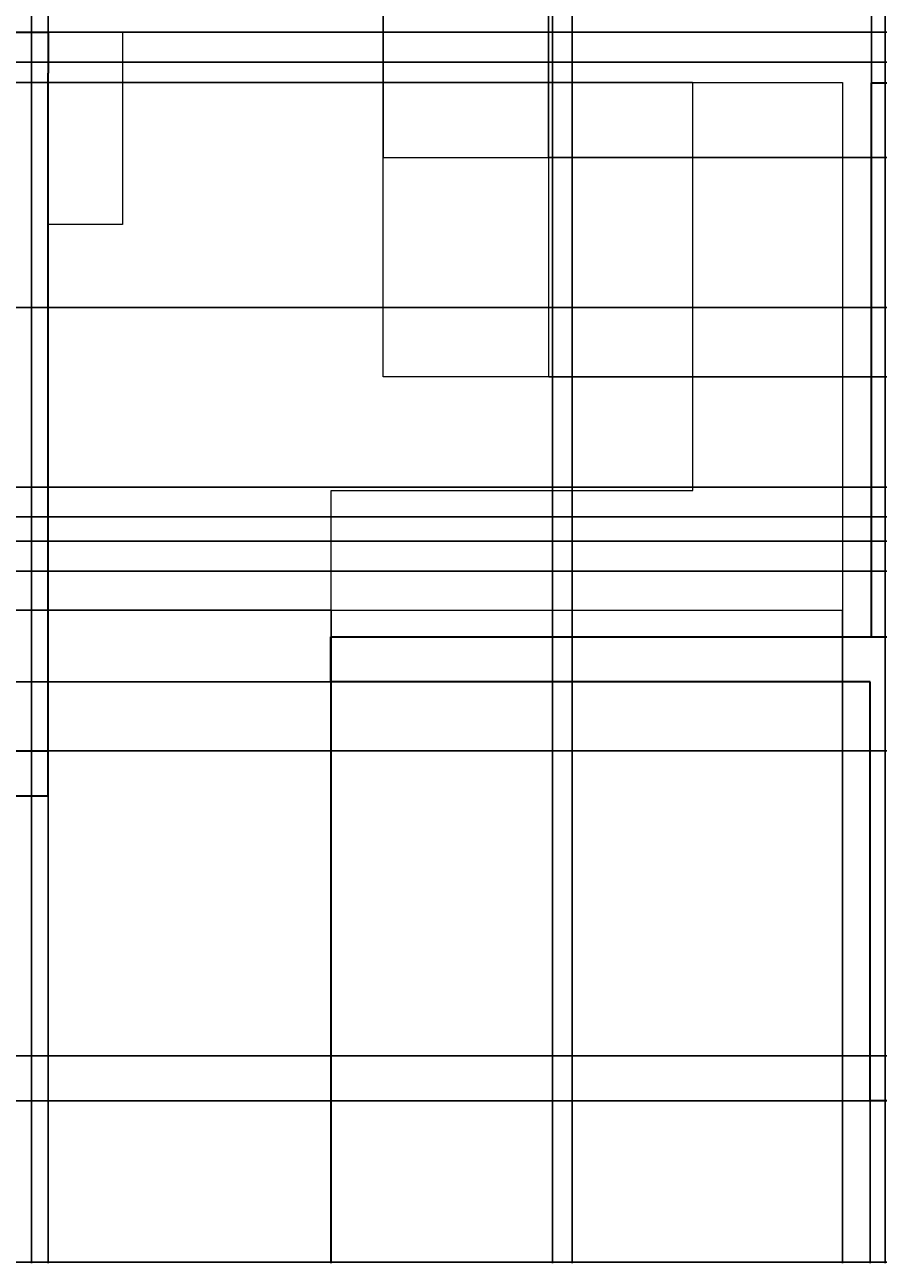
# Model space of a CAD drawing. Units: inches. Extents: x 1159 to 1869, y 2212 to 2738.
# Tile 3 of 5: x 1433 to 1604, y 2212 to 2460. Entities that reach past the tile are written whole.
import ezdxf

# ---------------------------------------------------------------- set-up
doc = ezdxf.new("R2010")
doc.units = ezdxf.units.IN
for name, color, linetype, lineweight in [('A-ANNO-DIMS', 2, 'Continuous', 18), ('A-FLOR-CASE', 30, 'Continuous', 18), ('A-FURN', 8, 'Continuous', 18), ('A-WALL', 7, 'Continuous', 35)]:
    doc.layers.add(name, color=color, linetype=linetype, lineweight=lineweight)
doc.styles.get("Standard").update_dxf_attribs({"font": 'arial.ttf'})
doc.dimstyles.get("Standard").update_dxf_attribs({"dimtxt": 0.18, "dimasz": 0.18, "dimexe": 0.18, "dimexo": 0.0625, "dimgap": 0.09, "dimtad": 0, "dimtih": 1, "dimtoh": 1, "dimdec": 4, "dimzin": 0, "dimdsep": 46, "dimtxsty": 'Standard', "dimcen": 0.09, "dimadec": 0, "dimazin": 0, "dimtfac": 1, "dimtdec": 4, "dimtofl": 0, "dimtmove": 0, "dimatfit": 3, "dimfxl": 1, "dimtolj": 1, "dimtzin": 0, "dimarcsym": 0})

# ---------------------------------------------------------------- blocks, each defined once
blk = doc.blocks.new('*D26')
at = {"layer": 'A-ANNO-DIMS', "color": 0, "lineweight": -2, "transparency": 16777216}
for p, q in [((1191.4, 2305.14), (1191.4, 2211.56)), ((1437.74, 2305.14), (1437.74, 2211.56)), ((1191.58, 2211.74), (1314.11, 2211.74)), ((1437.56, 2211.74), (1315.04, 2211.74))]:
    blk.add_line(p, q, dxfattribs=at)
at = {"layer": 'A-ANNO-DIMS', "color": 0, "transparency": 16777216}
for points in [[(1191.58, 2211.77), (1191.58, 2211.71), (1191.4, 2211.74)], [(1437.56, 2211.77), (1437.56, 2211.71), (1437.74, 2211.74)]]:
    blk.add_solid(points, dxfattribs=at)
at = {"layer": 'Defpoints', "color": 0, "transparency": 16777216}
for p in [(1191.4, 2305.21), (1437.74, 2305.21), (1437.74, 2211.74)]:
    blk.add_point(p, dxfattribs=at)
at = {"layer": 'A-ANNO-DIMS', "color": 0, "transparency": 16777216, "insert": (1314.57, 2211.74), "char_height": 0.18, "attachment_point": 5}
blk.add_mtext('\\A1;246.34', dxfattribs=at)
blk = doc.blocks.new('*D27')
at = {"layer": 'A-ANNO-DIMS', "color": 0, "lineweight": -2, "transparency": 16777216}
for p, q in [((1437.74, 2305.14), (1437.74, 2211.56)), ((1602.4, 2244.01), (1602.4, 2211.56)), ((1437.92, 2211.74), (1519.62, 2211.74)), ((1602.22, 2211.74), (1520.53, 2211.74))]:
    blk.add_line(p, q, dxfattribs=at)
at = {"layer": 'A-ANNO-DIMS', "color": 0, "transparency": 16777216}
for points in [[(1437.92, 2211.77), (1437.92, 2211.71), (1437.74, 2211.74)], [(1602.22, 2211.77), (1602.22, 2211.71), (1602.4, 2211.74)]]:
    blk.add_solid(points, dxfattribs=at)
at = {"layer": 'Defpoints', "color": 0, "transparency": 16777216}
for p in [(1437.74, 2305.21), (1602.4, 2244.08), (1602.4, 2211.74)]:
    blk.add_point(p, dxfattribs=at)
at = {"layer": 'A-ANNO-DIMS', "color": 0, "transparency": 16777216, "insert": (1520.07, 2211.74), "char_height": 0.18, "attachment_point": 5}
blk.add_mtext('\\A1;164.66', dxfattribs=at)
blk = doc.blocks.new('*D28')
at = {"layer": 'A-ANNO-DIMS', "color": 0, "lineweight": -2, "transparency": 16777216}
for p, q in [((1602.4, 2244.01), (1602.4, 2211.56)), ((1752.4, 2244.01), (1752.4, 2211.56)), ((1602.58, 2211.74), (1677.12, 2211.74)), ((1752.22, 2211.74), (1677.68, 2211.74))]:
    blk.add_line(p, q, dxfattribs=at)
at = {"layer": 'A-ANNO-DIMS', "color": 0, "transparency": 16777216}
for points in [[(1602.58, 2211.77), (1602.58, 2211.71), (1602.4, 2211.74)], [(1752.22, 2211.77), (1752.22, 2211.71), (1752.4, 2211.74)]]:
    blk.add_solid(points, dxfattribs=at)
at = {"layer": 'Defpoints', "color": 0, "transparency": 16777216}
for p in [(1602.4, 2244.08), (1752.4, 2244.08), (1752.4, 2211.74)]:
    blk.add_point(p, dxfattribs=at)
at = {"layer": 'A-ANNO-DIMS', "color": 0, "transparency": 16777216, "insert": (1677.4, 2211.74), "char_height": 0.18, "attachment_point": 5}
blk.add_mtext('\\A1;150', dxfattribs=at)
blk = doc.blocks.new('*D42')
at = {"layer": 'A-ANNO-DIMS', "color": 0, "lineweight": -2, "transparency": 16777216}
for p, q in [((1200.46, 2452.21), (1868.92, 2452.21)), ((1868.74, 2452.03), (1868.74, 2404.39)), ((1868.74, 2356.39), (1868.74, 2404.02)), ((1200.46, 2356.21), (1868.92, 2356.21))]:
    blk.add_line(p, q, dxfattribs=at)
at = {"layer": 'A-ANNO-DIMS', "color": 0, "transparency": 16777216}
for points in [[(1868.71, 2452.03), (1868.77, 2452.03), (1868.74, 2452.21)], [(1868.71, 2356.39), (1868.77, 2356.39), (1868.74, 2356.21)]]:
    blk.add_solid(points, dxfattribs=at)
at = {"layer": 'Defpoints', "color": 0, "transparency": 16777216}
for p in [(1200.4, 2452.21), (1868.74, 2452.21), (1200.4, 2356.21)]:
    blk.add_point(p, dxfattribs=at)
at = {"layer": 'A-ANNO-DIMS', "color": 0, "transparency": 16777216, "insert": (1868.74, 2404.21), "char_height": 0.18, "attachment_point": 5}
blk.add_mtext('\\A1;96', dxfattribs=at)
blk = doc.blocks.new('*D45')
at = {"layer": 'A-ANNO-DIMS', "color": 0, "lineweight": -2, "transparency": 16777216}
for p, q in [((1494.4, 2328.01), (1494.4, 2211.56)), ((1602.4, 2328.01), (1602.4, 2211.56)), ((1494.58, 2211.74), (1548.12, 2211.74)), ((1602.22, 2211.74), (1548.68, 2211.74))]:
    blk.add_line(p, q, dxfattribs=at)
at = {"layer": 'A-ANNO-DIMS', "color": 0, "transparency": 16777216}
for points in [[(1494.58, 2211.77), (1494.58, 2211.71), (1494.4, 2211.74)], [(1602.22, 2211.77), (1602.22, 2211.71), (1602.4, 2211.74)]]:
    blk.add_solid(points, dxfattribs=at)
at = {"layer": 'Defpoints', "color": 0, "transparency": 16777216}
for p in [(1494.4, 2328.08), (1602.4, 2328.08), (1602.4, 2211.74)]:
    blk.add_point(p, dxfattribs=at)
at = {"layer": 'A-ANNO-DIMS', "color": 0, "transparency": 16777216, "insert": (1548.4, 2211.74), "char_height": 0.18, "attachment_point": 5}
blk.add_mtext('\\A1;108', dxfattribs=at)
blk = doc.blocks.new('*D46')
at = {"layer": 'A-ANNO-DIMS', "color": 0, "lineweight": -2, "transparency": 16777216}
for p, q in [((1602.34, 2328.08), (1158.88, 2328.08)), ((1159.06, 2327.9), (1159.06, 2286.26)), ((1159.06, 2244.26), (1159.06, 2285.89)), ((1602.34, 2244.08), (1158.88, 2244.08))]:
    blk.add_line(p, q, dxfattribs=at)
at = {"layer": 'A-ANNO-DIMS', "color": 0, "transparency": 16777216}
for points in [[(1159.03, 2327.9), (1159.09, 2327.9), (1159.06, 2328.08)], [(1159.03, 2244.26), (1159.09, 2244.26), (1159.06, 2244.08)]]:
    blk.add_solid(points, dxfattribs=at)
at = {"layer": 'Defpoints', "color": 0, "transparency": 16777216}
for p in [(1159.06, 2328.08), (1602.4, 2328.08), (1602.4, 2244.08)]:
    blk.add_point(p, dxfattribs=at)
at = {"layer": 'A-ANNO-DIMS', "color": 0, "transparency": 16777216, "insert": (1159.06, 2286.08), "char_height": 0.18, "attachment_point": 5}
blk.add_mtext('\\A1;84', dxfattribs=at)
blk = doc.blocks.new('*D48')
at = {"layer": 'A-ANNO-DIMS', "color": 0, "lineweight": -2, "transparency": 16777216}
for p, q in [((1437.74, 2458.27), (1437.74, 2738.15)), ((1437.92, 2737.97), (1519.76, 2737.97)), ((1602.5, 2737.97), (1520.67, 2737.97)), ((1602.68, 2448.14), (1602.68, 2738.15))]:
    blk.add_line(p, q, dxfattribs=at)
at = {"layer": 'A-ANNO-DIMS', "color": 0, "transparency": 16777216}
for points in [[(1437.92, 2738), (1437.92, 2737.94), (1437.74, 2737.97)], [(1602.5, 2738), (1602.5, 2737.94), (1602.68, 2737.97)]]:
    blk.add_solid(points, dxfattribs=at)
at = {"layer": 'Defpoints', "color": 0, "transparency": 16777216}
for p in [(1602.68, 2737.97), (1437.74, 2458.21), (1602.68, 2448.08)]:
    blk.add_point(p, dxfattribs=at)
at = {"layer": 'A-ANNO-DIMS', "color": 0, "transparency": 16777216, "insert": (1520.21, 2737.97), "char_height": 0.18, "attachment_point": 5}
blk.add_mtext('\\A1;164.94', dxfattribs=at)
blk = doc.blocks.new('*D53')
at = {"layer": 'A-ANNO-DIMS', "color": 0, "lineweight": -2, "transparency": 16777216}
for p, q in [((1425.46, 2504.63), (1868.92, 2504.63)), ((1868.74, 2504.45), (1868.74, 2481.6)), ((1868.74, 2458.39), (1868.74, 2481.24)), ((1428.81, 2458.21), (1868.92, 2458.21))]:
    blk.add_line(p, q, dxfattribs=at)
at = {"layer": 'A-ANNO-DIMS', "color": 0, "transparency": 16777216}
for points in [[(1868.71, 2504.45), (1868.77, 2504.45), (1868.74, 2504.63)], [(1868.71, 2458.39), (1868.77, 2458.39), (1868.74, 2458.21)]]:
    blk.add_solid(points, dxfattribs=at)
at = {"layer": 'Defpoints', "color": 0, "transparency": 16777216}
for p in [(1425.4, 2504.63), (1868.74, 2504.63), (1428.74, 2458.21)]:
    blk.add_point(p, dxfattribs=at)
at = {"layer": 'A-ANNO-DIMS', "color": 0, "transparency": 16777216, "insert": (1868.74, 2481.42), "char_height": 0.18, "attachment_point": 5}
blk.add_mtext('\\A1;46.42', dxfattribs=at)
blk = doc.blocks.new('*D54')
at = {"layer": 'A-ANNO-DIMS', "color": 0, "lineweight": -2, "transparency": 16777216}
for p, q in [((1437.68, 2305.21), (1158.88, 2305.21)), ((1159.06, 2305.03), (1159.06, 2274.82)), ((1159.06, 2244.26), (1159.06, 2274.46)), ((1602.34, 2244.08), (1158.88, 2244.08))]:
    blk.add_line(p, q, dxfattribs=at)
at = {"layer": 'A-ANNO-DIMS', "color": 0, "transparency": 16777216}
for points in [[(1159.03, 2305.03), (1159.09, 2305.03), (1159.06, 2305.21)], [(1159.03, 2244.26), (1159.09, 2244.26), (1159.06, 2244.08)]]:
    blk.add_solid(points, dxfattribs=at)
at = {"layer": 'Defpoints', "color": 0, "transparency": 16777216}
for p in [(1437.74, 2305.21), (1159.06, 2244.08), (1602.4, 2244.08)]:
    blk.add_point(p, dxfattribs=at)
at = {"layer": 'A-ANNO-DIMS', "color": 0, "transparency": 16777216, "insert": (1159.06, 2274.64), "char_height": 0.18, "attachment_point": 5}
blk.add_mtext('\\A1;61.13', dxfattribs=at)
blk = doc.blocks.new('*D55')
at = {"layer": 'A-ANNO-DIMS', "color": 0, "lineweight": -2, "transparency": 16777216}
for p, q in [((1494.46, 2342.31), (1494.46, 2211.56)), ((1596.87, 2342.31), (1596.87, 2211.56)), ((1494.64, 2211.74), (1545.28, 2211.74)), ((1596.69, 2211.74), (1546.05, 2211.74))]:
    blk.add_line(p, q, dxfattribs=at)
at = {"layer": 'A-ANNO-DIMS', "color": 0, "transparency": 16777216}
for points in [[(1494.64, 2211.77), (1494.64, 2211.71), (1494.46, 2211.74)], [(1596.69, 2211.77), (1596.69, 2211.71), (1596.87, 2211.74)]]:
    blk.add_solid(points, dxfattribs=at)
at = {"layer": 'Defpoints', "color": 0, "transparency": 16777216}
for p in [(1494.46, 2342.38), (1596.87, 2342.38), (1596.87, 2211.74)]:
    blk.add_point(p, dxfattribs=at)
at = {"layer": 'A-ANNO-DIMS', "color": 0, "transparency": 16777216, "insert": (1545.66, 2211.74), "char_height": 0.18, "attachment_point": 5}
blk.add_mtext('\\A1;102.4', dxfattribs=at)
blk = doc.blocks.new('*D56')
at = {"layer": 'A-ANNO-DIMS', "color": 0, "lineweight": -2, "transparency": 16777216}
for p, q in [((1566.83, 2448.11), (1158.88, 2448.11)), ((1159.06, 2447.93), (1159.06, 2395.42)), ((1159.06, 2342.56), (1159.06, 2395.06)), ((1494.4, 2342.38), (1158.88, 2342.38))]:
    blk.add_line(p, q, dxfattribs=at)
at = {"layer": 'A-ANNO-DIMS', "color": 0, "transparency": 16777216}
for points in [[(1159.03, 2447.93), (1159.09, 2447.93), (1159.06, 2448.11)], [(1159.03, 2342.56), (1159.09, 2342.56), (1159.06, 2342.38)]]:
    blk.add_solid(points, dxfattribs=at)
at = {"layer": 'Defpoints', "color": 0, "transparency": 16777216}
for p in [(1566.9, 2448.11), (1159.06, 2342.38), (1494.46, 2342.38)]:
    blk.add_point(p, dxfattribs=at)
at = {"layer": 'A-ANNO-DIMS', "color": 0, "transparency": 16777216, "insert": (1159.06, 2395.24), "char_height": 0.18, "attachment_point": 5}
blk.add_mtext('\\A1;105.73', dxfattribs=at)
blk = doc.blocks.new('*D57')
at = {"layer": 'A-ANNO-DIMS', "color": 0, "lineweight": -2, "transparency": 16777216}
for p, q in [((1504.87, 2433.16), (1504.87, 2738.15)), ((1505.05, 2737.97), (1521.04, 2737.97)), ((1537.79, 2737.97), (1521.8, 2737.97)), ((1537.97, 2433.16), (1537.97, 2738.15))]:
    blk.add_line(p, q, dxfattribs=at)
at = {"layer": 'A-ANNO-DIMS', "color": 0, "transparency": 16777216}
for points in [[(1505.05, 2738), (1505.05, 2737.94), (1504.87, 2737.97)], [(1537.79, 2738), (1537.79, 2737.94), (1537.97, 2737.97)]]:
    blk.add_solid(points, dxfattribs=at)
at = {"layer": 'Defpoints', "color": 0, "transparency": 16777216}
for p in [(1537.97, 2737.97), (1504.87, 2433.09), (1537.97, 2433.09)]:
    blk.add_point(p, dxfattribs=at)
at = {"layer": 'A-ANNO-DIMS', "color": 0, "transparency": 16777216, "insert": (1521.42, 2737.97), "char_height": 0.18, "attachment_point": 5}
blk.add_mtext('\\A1;33.11', dxfattribs=at)
blk = doc.blocks.new('*D58')
at = {"layer": 'A-ANNO-DIMS', "color": 0, "lineweight": -2, "transparency": 16777216}
for p, q in [((1538.03, 2433.09), (1868.92, 2433.09)), ((1868.74, 2432.91), (1868.74, 2411.32)), ((1868.74, 2389.36), (1868.74, 2410.95)), ((1538.03, 2389.18), (1868.92, 2389.18))]:
    blk.add_line(p, q, dxfattribs=at)
at = {"layer": 'A-ANNO-DIMS', "color": 0, "transparency": 16777216}
for points in [[(1868.71, 2432.91), (1868.77, 2432.91), (1868.74, 2433.09)], [(1868.71, 2389.36), (1868.77, 2389.36), (1868.74, 2389.18)]]:
    blk.add_solid(points, dxfattribs=at)
at = {"layer": 'Defpoints', "color": 0, "transparency": 16777216}
for p in [(1537.97, 2433.09), (1868.74, 2433.09), (1537.97, 2389.18)]:
    blk.add_point(p, dxfattribs=at)
at = {"layer": 'A-ANNO-DIMS', "color": 0, "transparency": 16777216, "insert": (1868.74, 2411.14), "char_height": 0.18, "attachment_point": 5}
blk.add_mtext('\\A1;43.92', dxfattribs=at)
blk = doc.blocks.new('*D64')
at = {"layer": 'A-ANNO-DIMS', "color": 0, "lineweight": -2, "transparency": 16777216}
for p, q in [((1434.4, 2660.2), (1434.4, 2211.56)), ((1538.82, 2660.2), (1538.82, 2211.56)), ((1434.58, 2211.74), (1486.15, 2211.74)), ((1538.64, 2211.74), (1487.06, 2211.74))]:
    blk.add_line(p, q, dxfattribs=at)
at = {"layer": 'A-ANNO-DIMS', "color": 0, "transparency": 16777216}
for points in [[(1434.58, 2211.77), (1434.58, 2211.71), (1434.4, 2211.74)], [(1538.64, 2211.77), (1538.64, 2211.71), (1538.82, 2211.74)]]:
    blk.add_solid(points, dxfattribs=at)
at = {"layer": 'Defpoints', "color": 0, "transparency": 16777216}
for p in [(1434.4, 2660.26), (1538.82, 2660.26), (1434.4, 2211.74)]:
    blk.add_point(p, dxfattribs=at)
at = {"layer": 'A-ANNO-DIMS', "color": 0, "transparency": 16777216, "insert": (1486.61, 2211.74), "char_height": 0.18, "attachment_point": 5}
blk.add_mtext('\\A1;104.42', dxfattribs=at)
blk = doc.blocks.new('*D65')
at = {"layer": 'A-ANNO-DIMS', "color": 0, "lineweight": -2, "transparency": 16777216}
for p, q in [((1542.76, 2504.57), (1542.76, 2211.56)), ((1605.4, 2504.57), (1605.4, 2211.56)), ((1542.94, 2211.74), (1573.69, 2211.74)), ((1605.22, 2211.74), (1574.48, 2211.74))]:
    blk.add_line(p, q, dxfattribs=at)
at = {"layer": 'A-ANNO-DIMS', "color": 0, "transparency": 16777216}
for points in [[(1542.94, 2211.77), (1542.94, 2211.71), (1542.76, 2211.74)], [(1605.22, 2211.77), (1605.22, 2211.71), (1605.4, 2211.74)]]:
    blk.add_solid(points, dxfattribs=at)
at = {"layer": 'Defpoints', "color": 0, "transparency": 16777216}
for p in [(1542.76, 2504.63), (1605.4, 2504.63), (1605.4, 2211.74)]:
    blk.add_point(p, dxfattribs=at)
at = {"layer": 'A-ANNO-DIMS', "color": 0, "transparency": 16777216, "insert": (1574.08, 2211.74), "char_height": 0.18, "attachment_point": 5}
blk.add_mtext('\\A1;62.64', dxfattribs=at)
blk = doc.blocks.new('*D67')
at = {"layer": 'A-ANNO-DIMS', "color": 0, "lineweight": -2, "transparency": 16777216}
for p, q in [((1665.34, 2403.08), (1158.88, 2403.08)), ((1159.06, 2402.9), (1159.06, 2385.26)), ((1159.06, 2367.26), (1159.06, 2384.89)), ((1665.34, 2367.08), (1158.88, 2367.08))]:
    blk.add_line(p, q, dxfattribs=at)
at = {"layer": 'A-ANNO-DIMS', "color": 0, "transparency": 16777216}
for points in [[(1159.03, 2402.9), (1159.09, 2402.9), (1159.06, 2403.08)], [(1159.03, 2367.26), (1159.09, 2367.26), (1159.06, 2367.08)]]:
    blk.add_solid(points, dxfattribs=at)
at = {"layer": 'Defpoints', "color": 0, "transparency": 16777216}
for p in [(1159.06, 2403.08), (1665.4, 2403.08), (1665.4, 2367.08)]:
    blk.add_point(p, dxfattribs=at)
at = {"layer": 'A-ANNO-DIMS', "color": 0, "transparency": 16777216, "insert": (1159.06, 2385.08), "char_height": 0.18, "attachment_point": 5}
blk.add_mtext('\\A1;36', dxfattribs=at)
blk = doc.blocks.new('*D74')
at = {"layer": 'A-ANNO-DIMS', "color": 0, "lineweight": -2, "transparency": 16777216}
for p, q in [((1743.34, 2361.08), (1158.88, 2361.08)), ((1159.06, 2360.9), (1159.06, 2307.26)), ((1159.06, 2253.26), (1159.06, 2306.89)), ((1743.34, 2253.08), (1158.88, 2253.08))]:
    blk.add_line(p, q, dxfattribs=at)
at = {"layer": 'A-ANNO-DIMS', "color": 0, "transparency": 16777216}
for points in [[(1159.03, 2360.9), (1159.09, 2360.9), (1159.06, 2361.08)], [(1159.03, 2253.26), (1159.09, 2253.26), (1159.06, 2253.08)]]:
    blk.add_solid(points, dxfattribs=at)
at = {"layer": 'Defpoints', "color": 0, "transparency": 16777216}
for p in [(1159.06, 2361.08), (1743.4, 2361.08), (1743.4, 2253.08)]:
    blk.add_point(p, dxfattribs=at)
at = {"layer": 'A-ANNO-DIMS', "color": 0, "transparency": 16777216, "insert": (1159.06, 2307.08), "char_height": 0.18, "attachment_point": 5}
blk.add_mtext('\\A1;108', dxfattribs=at)
blk = doc.blocks.new('*D75')
at = {"layer": 'A-ANNO-DIMS', "color": 0, "lineweight": -2, "transparency": 16777216}
for p, q in [((1227.43, 2350.21), (1868.92, 2350.21)), ((1868.74, 2350.03), (1868.74, 2332.39)), ((1868.74, 2314.39), (1868.74, 2332.02)), ((1227.43, 2314.21), (1868.92, 2314.21))]:
    blk.add_line(p, q, dxfattribs=at)
at = {"layer": 'A-ANNO-DIMS', "color": 0, "transparency": 16777216}
for points in [[(1868.71, 2350.03), (1868.77, 2350.03), (1868.74, 2350.21)], [(1868.71, 2314.39), (1868.77, 2314.39), (1868.74, 2314.21)]]:
    blk.add_solid(points, dxfattribs=at)
at = {"layer": 'Defpoints', "color": 0, "transparency": 16777216}
for p in [(1227.37, 2350.21), (1868.74, 2350.21), (1227.37, 2314.21)]:
    blk.add_point(p, dxfattribs=at)
at = {"layer": 'A-ANNO-DIMS', "color": 0, "transparency": 16777216, "insert": (1868.74, 2332.21), "char_height": 0.18, "attachment_point": 5}
blk.add_mtext('\\A1;36', dxfattribs=at)

msp = doc.modelspace()

# ---------------------------------------------------------------- linework, layer by layer
at = {"layer": 'A-FLOR-CASE'}
for p, q in [((1437.7443, 2458.2064), (1452.6751, 2458.2064)), ((1452.6751, 2458.2064), (1452.6751, 2419.6842)), ((1452.6751, 2419.6842), (1437.7443, 2419.6842))]:
    msp.add_line(p, q, dxfattribs=at)
at = {"layer": 'A-FURN'}
for p, q in [((1566.895, 2366.3753), (1566.895, 2448.1096)), ((1566.895, 2448.1096), (1596.8651, 2448.1096)), ((1596.8651, 2448.1096), (1596.8651, 2342.3753)), ((1494.4613, 2342.3753), (1494.4613, 2366.3753)), ((1494.4613, 2366.3753), (1566.895, 2366.3753)), ((1596.8651, 2342.3753), (1494.4613, 2342.3753))]:
    msp.add_line(p, q, dxfattribs=at)
msp.add_lwpolyline([(1504.8654, 2433.0936), (1537.9722, 2433.0936), (1537.9722, 2389.1774), (1504.8654, 2389.1774)], close=True, dxfattribs=at)
at = {"layer": 'A-WALL'}
for p, q in [((1428.7443, 2458.2064), (1437.7443, 2458.2064)), ((1437.7443, 2458.2064), (1437.7443, 2449.977)), ((1437.7443, 2314.2064), (1437.7443, 2449.977)), ((1602.6806, 2337.0757), (1602.6806, 2448.0757)), ((1602.6806, 2448.0757), (1632.6806, 2448.0757)), ((1494.4011, 2328.0757), (1494.4011, 2337.0757)), ((1494.4011, 2337.0757), (1611.4011, 2337.0757)), ((1602.4011, 2328.0757), (1494.4011, 2328.0757)), ((1602.4011, 2244.0757), (1602.4011, 2328.0757)), ((1200.4011, 2314.2064), (1437.7443, 2314.2064)), ((1437.7443, 2305.2064), (1437.7443, 2314.2064)), ((1191.4011, 2305.2064), (1437.7443, 2305.2064)), ((1614.4011, 2244.0757), (1602.4011, 2244.0757))]:
    msp.add_line(p, q, dxfattribs=at)

# ---------------------------------------------------------------- dimensions: what is measured, and where the dimension line sits
at = {"layer": 'A-ANNO-DIMS'}
for base, p1, p2, override, picture, middle in [((1602.6806, 2737.9679), (1437.7443, 2458.2064), (1602.6806, 2448.0757), {"dimdec": 2, "dimlfac": 1, "dimrnd": 0, "dimzin": 0, "dimdsep": 46, "dimlunit": 2}, '*D48', (1520.2124, 2737.9679)), ((1537.9722, 2737.9679), (1504.8654, 2433.0936), (1537.9722, 2433.0936), {"dimdec": 2, "dimlfac": 1, "dimrnd": 0, "dimzin": 0, "dimdsep": 46, "dimlunit": 2}, '*D57', (1521.4188, 2737.9679)), ((1434.4011, 2211.7357), (1538.817, 2660.2597), (1434.4011, 2660.2597), {"dimdec": 2, "dimlfac": 1, "dimrnd": 0, "dimzin": 0, "dimdsep": 46, "dimlunit": 2}, '*D64', (1486.6091, 2211.7357)), ((1605.4011, 2211.7357), (1542.764, 2504.6279), (1605.4011, 2504.6279), {"dimdec": 2, "dimlfac": 1, "dimrnd": 0, "dimzin": 0, "dimdsep": 46, "dimlunit": 2}, '*D65', (1574.0826, 2211.7357)), ((1596.8651, 2211.7357), (1494.4613, 2342.3753), (1596.8651, 2342.3753), {"dimdec": 1, "dimlfac": 1, "dimrnd": 0, "dimzin": 0, "dimdsep": 46, "dimlunit": 2}, '*D55', (1545.6632, 2211.7357)), ((1602.4011, 2211.7357), (1494.4011, 2328.0757), (1602.4011, 2328.0757), {"dimdec": 0, "dimlfac": 1, "dimrnd": 0, "dimzin": 0, "dimdsep": 46, "dimlunit": 2}, '*D45', (1548.4011, 2211.7357)), ((1437.7443, 2211.7357), (1191.4011, 2305.2064), (1437.7443, 2305.2064), {"dimdec": 2, "dimlfac": 1, "dimrnd": 0, "dimzin": 0, "dimdsep": 46, "dimlunit": 2}, '*D26', (1314.5727, 2211.7357)), ((1602.4011, 2211.7357), (1437.7443, 2305.2064), (1602.4011, 2244.0757), {"dimdec": 2, "dimlfac": 1, "dimrnd": 0, "dimzin": 0, "dimdsep": 46, "dimlunit": 2}, '*D27', (1520.0727, 2211.7357)), ((1752.4011, 2211.7357), (1602.4011, 2244.0757), (1752.4011, 2244.0757), {"dimdec": 0, "dimlfac": 1, "dimrnd": 0, "dimzin": 0, "dimdsep": 46, "dimlunit": 2}, '*D28', (1677.4011, 2211.7357))]:
    dim = msp.add_linear_dim(base=base, p1=p1, p2=p2, dimstyle='Standard', override=override, dxfattribs=at)
    dim.commit()
    dim.dimension.update_dxf_attribs({"geometry": picture, "text_midpoint": middle})
for base, p1, p2, override, picture, middle in [((1868.7411, 2504.6279), (1428.7443, 2458.2064), (1425.4011, 2504.6279), {"dimdec": 2, "dimlfac": 1, "dimrnd": 0, "dimzin": 0, "dimdsep": 46, "dimlunit": 2}, '*D53', (1868.7411, 2481.4172)), ((1868.7411, 2452.2064), (1200.4011, 2356.2064), (1200.4011, 2452.2064), {"dimdec": 0, "dimlfac": 1, "dimrnd": 0, "dimzin": 0, "dimdsep": 46, "dimlunit": 2}, '*D42', (1868.7411, 2404.2064)), ((1159.0611, 2342.3753), (1566.895, 2448.1096), (1494.4613, 2342.3753), {"dimdec": 2, "dimlfac": 1, "dimrnd": 0, "dimzin": 0, "dimdsep": 46, "dimlunit": 2}, '*D56', (1159.0611, 2395.2425)), ((1868.7411, 2433.0936), (1537.9722, 2389.1774), (1537.9722, 2433.0936), {"dimdec": 2, "dimlfac": 1, "dimrnd": 0, "dimzin": 0, "dimdsep": 46, "dimlunit": 2}, '*D58', (1868.7411, 2411.1355)), ((1159.0611, 2403.0757), (1665.4011, 2367.0757), (1665.4011, 2403.0757), {"dimdec": 0, "dimlfac": 1, "dimrnd": 0, "dimzin": 0, "dimdsep": 46, "dimlunit": 2}, '*D67', (1159.0611, 2385.0757)), ((1159.0611, 2361.0757), (1743.4011, 2253.0757), (1743.4011, 2361.0757), {"dimdec": 0, "dimlfac": 1, "dimrnd": 0, "dimzin": 0, "dimdsep": 46, "dimlunit": 2}, '*D74', (1159.0611, 2307.0757)), ((1868.7411, 2350.2064), (1227.3685, 2314.2064), (1227.3685, 2350.2064), {"dimdec": 0, "dimlfac": 1, "dimrnd": 0, "dimzin": 0, "dimdsep": 46, "dimlunit": 2}, '*D75', (1868.7411, 2332.2064)), ((1159.0611, 2328.0757), (1602.4011, 2244.0757), (1602.4011, 2328.0757), {"dimdec": 0, "dimlfac": 1, "dimrnd": 0, "dimzin": 0, "dimdsep": 46, "dimlunit": 2}, '*D46', (1159.0611, 2286.0757)), ((1159.0611, 2244.0757), (1437.7443, 2305.2064), (1602.4011, 2244.0757), {"dimdec": 2, "dimlfac": 1, "dimrnd": 0, "dimzin": 0, "dimdsep": 46, "dimlunit": 2}, '*D54', (1159.0611, 2274.6411))]:
    dim = msp.add_linear_dim(base=base, p1=p1, p2=p2, angle=90, dimstyle='Standard', override=override, dxfattribs=at)
    dim.commit()
    dim.dimension.update_dxf_attribs({"geometry": picture, "text_midpoint": middle})

doc.saveas('drawing.dxf')
